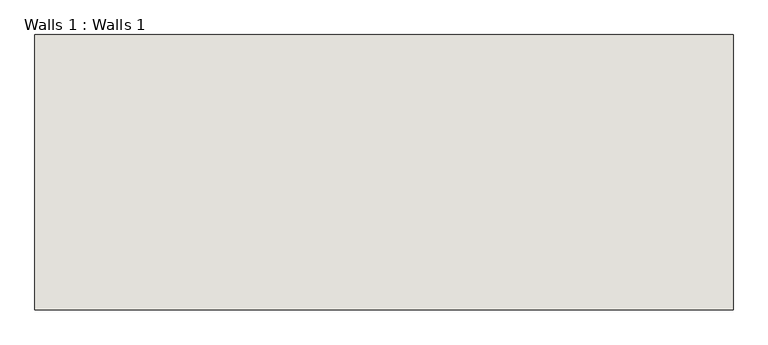
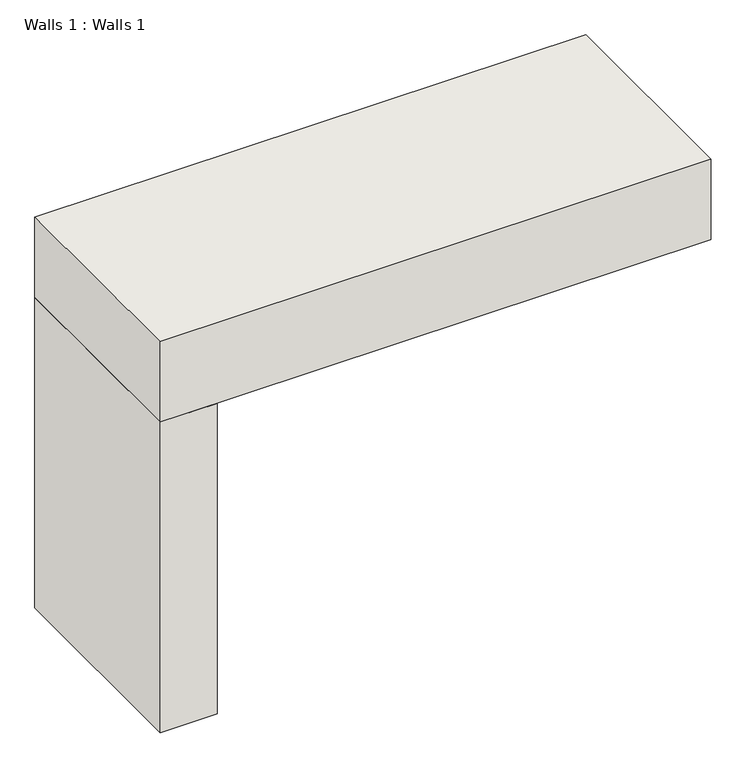
"""IFC4 building model written with IfcOpenShell, lengths in millimetres: wall geometry, Walls 1 : Walls 1."""

from ifc_helpers import new_model, si_unit, frame, origin, place, context, project, spatial, polyline, outline, extrude, source, transform, mapped, element, save


def walls_1_walls_1_cd62c845(model_context):
    return source(origin(), model_context, "Body", "SweptSolid", [
        extrude(outline(polyline([(-9729.3009562, 516.1148832), (-9729.3009562, 2270.9425923), (-9272.1009562, 2270.9425923), (-9272.1009562, 516.1148832), (-9729.3009562, 516.1148832)])), frame((0.0, 0.0, 7620.0), z_axis=(0.0, 0.0, 1.0), x_axis=(1.0, 0.0, 0.0)), (0.0, 0.0, 1.0), 2650.3479799),
        extrude(outline(polyline([(-9729.3009562, 518.3425923), (-9729.3009562, 2270.9425923), (-5281.411895, 2270.9425923), (-5281.411895, 518.3425923), (-9729.3009562, 518.3425923)])), frame((0.0, 0.0, 10270.3479799), z_axis=(0.0, 0.0, 1.0), x_axis=(1.0, 0.0, 0.0)), (0.0, 0.0, 1.0), 685.8),
    ])


if __name__ == "__main__":
    model = new_model("IFC4")
    model_context = context("Model", 3, world=origin())
    ifc_project = project(units=[si_unit("LENGTHUNIT", "METRE", prefix="MILLI")], contexts=[model_context])
    site = spatial("IfcSite", under=ifc_project)
    building = spatial("IfcBuilding", under=site)
    placement = place(None, origin())
    walls_1_walls_1_shape = walls_1_walls_1_cd62c845(model_context)
    element("IfcWall", 1, ObjectType="Walls 1 : Walls 1", at=placement, inside=building, context=model_context, shape_type="MappedRepresentation", body=[
        mapped(walls_1_walls_1_shape, transform((0.0, 0.0, 0.0), x_axis=(1.0, 0.0, 0.0), y_axis=(0.0, 1.0, 0.0), z_axis=(0.0, 0.0, 1.0))),
    ])
    save(model, "model.ifc")

# Revit data of these elements
# Element 1 (IfcWall, "Walls 1 : Walls 1")
#   Materials on its faces: "Default Wall"
# Materials
#   "Default Wall": colour RGB 128 128 128, transparency 0
